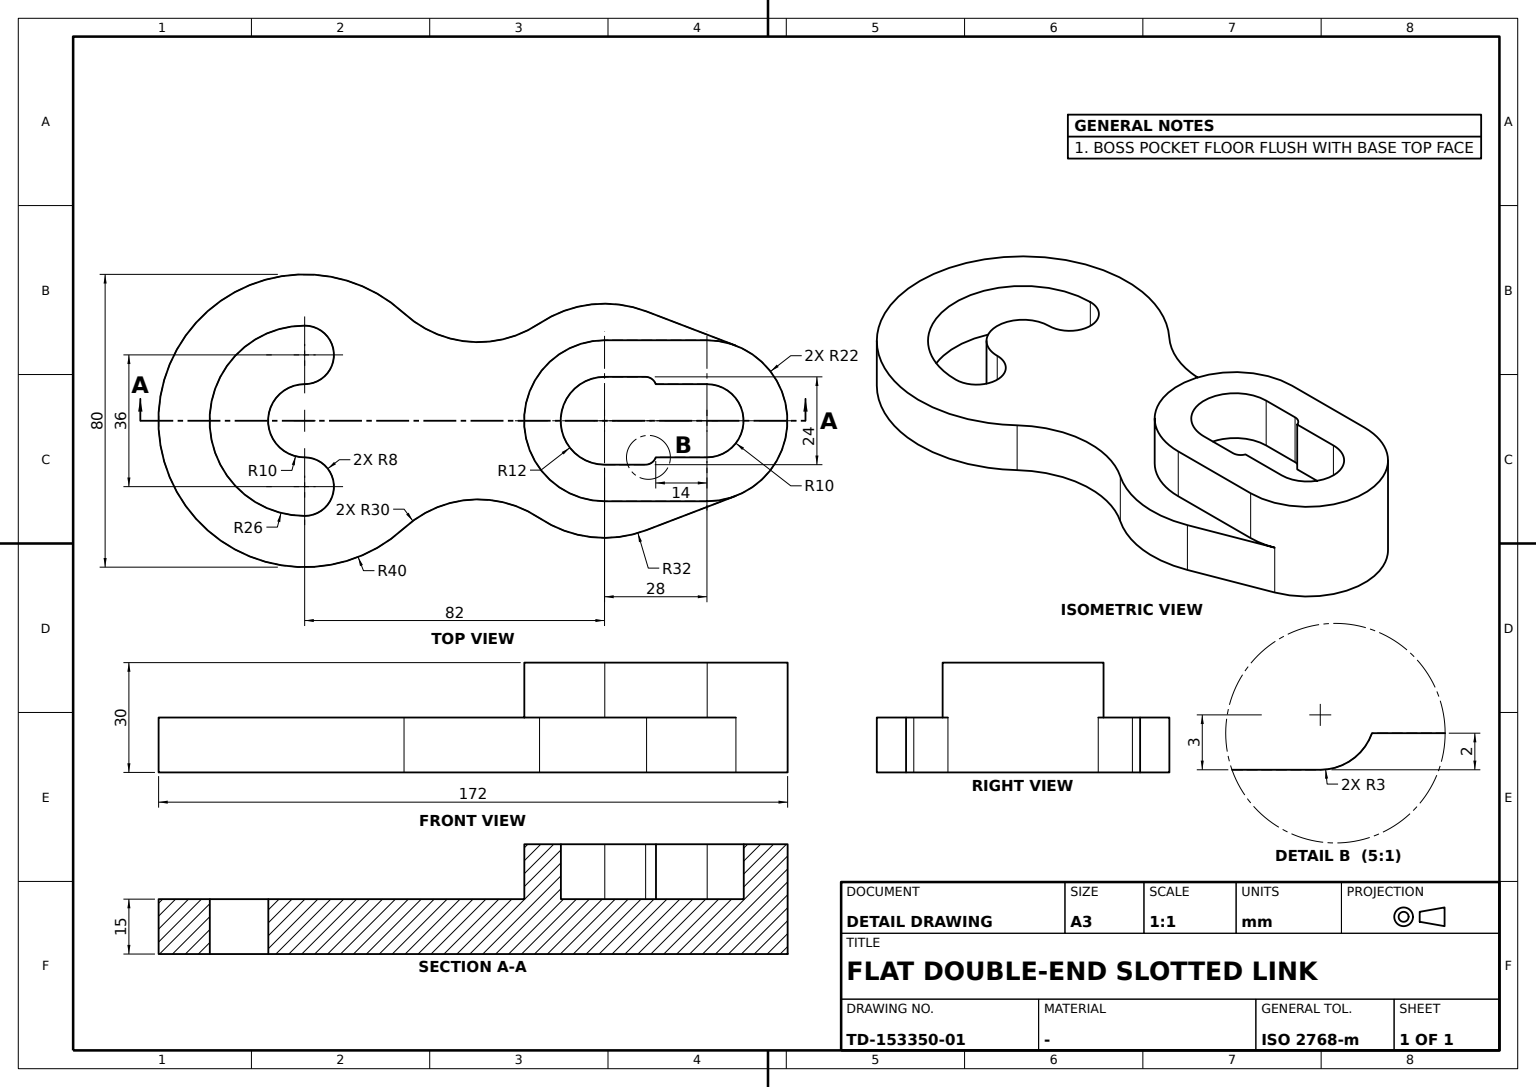
CATIA V5 part; units mm, degrees
sketch "Sketch1" plane through (0, 0, 0) normal (0, 0, 1) x (1, 0, 0)
  arc A0 (-29.4135, 27.108) -> (29.4135, 27.108) centre (0, 0) ccw
  arc A1 (26.5671, 64.1621) -> (29.8896, 93.4286) centre (0, 82) ccw
  point P0 (0, 82)
  arc A2 (26.5671, 64.1621) -> (29.4135, 27.108) centre (51.4737, 47.439) ccw
  arc A3 (-29.4135, 27.108) -> (-26.5671, 64.1621) centre (-51.4737, 47.439) ccw
  arc A4 (20.5491, 117.8571) -> (-20.5491, 117.8571) centre (0, 110) ccw
  point P1 (0, 110)
  line L0 (29.8896, 93.4286) -> (20.5491, 117.8571)
  line L1 (-29.8896, 93.4286) -> (-20.5491, 117.8571)
  point P2 (-29.8896, 93.4286)
  arc A5 (-29.8896, 93.4286) -> (-26.5671, 64.1621) centre (0, 82) ccw
  arc A6 (-18, 0) -> (18, 0) centre (0, 0) ccw construction
  point P3 (0, 0)
  point P4 (-18, 0)
  point P5 (18, 0)
  arc A7 (-26, 0) -> (-10, 0) centre (-18, 0) cw
  arc A8 (10, 0) -> (26, 0) centre (18, 0) cw
  arc A9 (-10, 0) -> (10, 0) centre (0, 0) ccw
  arc A10 (26, 0) -> (-26, 0) centre (0, 0) cw
  dimension "radius A0" = 40
  dimension "radius A1" = 32
  dimension "distance x axis P0" = 82
  dimension "radius A2" = 30
  dimension "radius A3" = 30
  dimension "radius A4" = 22
  dimension "distance P0 P1" = 28
  dimension "radius A8" = 8
  dimension "distance P5 y axis" = 18
  dimension "distance y axis P4" = 18
  constraint coincidence P0 y-axis
  constraint coincidence P1 y-axis
  constraint coincidence P2 A1
  constraint coincidence A1 A5
  constraint coincidence P3 x-axis
  constraint coincidence P4 x-axis
  constraint coincidence P5 x-axis
  constraint tangency A2 A0
  constraint tangency A2 A1
  constraint tangency A3 A0
  constraint tangency A3 A1
  constraint tangency L0 A4
  constraint tangency L0 A1
  constraint tangency L1 A4
  constraint tangency L1 A1
  constraint tangency A9 A8
  constraint tangency A8 A10
  constraint tangency A10 A7
  constraint tangency A7 A9
  constraint concentricity A9 P3
  constraint concentricity A10 P3
extrude "Pad1" add sketch "Sketch1" against normal blind 15
sketch "Sketch2" plane through (0, 0, 0) normal (0, 0, 1) x (1, 0, 0)
  line L0 (0, 110) -> (0, 82) construction
  point P0 (0, 110)
  line L1 (22, 110) -> (22, 82)
  line L2 (-22, 82) -> (-22, 110)
  arc A0 (22, 82) -> (-22, 82) centre (0, 82) cw
  arc A1 (-22, 110) -> (22, 110) centre (0, 110) cw
  arc A2 (20.5491, 117.8571) -> (-20.5491, 117.8571) centre (0, 110) ccw construction
  arc A3 (-12, 82) -> (12, 82) centre (0, 82) ccw
  arc A4 (10, 110) -> (-10, 110) centre (0, 110) ccw
  line L3 (10, 110) -> (10, 96)
  point P1 (10, 110)
  point P2 (10, 96)
  line L4 (12, 82) -> (12, 93.1716)
  point P3 (12, 82)
  point P4 (12, 93.1716)
  arc A5 (12, 93.1716) -> (10, 96) centre (9, 93.1716) ccw
  point P5 (-12, 93.1716)
  point P6 (-12, 82)
  line L5 (-12, 82) -> (-12, 93.1716)
  point P7 (-10, 96)
  arc A6 (-12, 93.1716) -> (-10, 96) centre (-9, 93.1716) cw
  point P8 (-10, 110)
  line L6 (-10, 110) -> (-10, 96)
  point P9 (12, 82)
  dimension "radius A1" = 22
  dimension "length L0" = 28
  dimension "radius A0" = 22
  dimension "radius A3" = 12
  dimension "radius A4" = 10
  dimension "length L3" = 14
  dimension "radius A5" = 3
  constraint coincidence P0 y-axis
  constraint coincidence P3 A3
  constraint coincidence L4 P9
  constraint coincidence P3 P9
  constraint vertical L0 y-axis
  constraint tangency A0 L1
  constraint tangency A1 L1
  constraint tangency A0 L2
  constraint tangency A1 L2
  constraint tangency L3 A4
  constraint tangency L4 A3
  constraint tangency A5 L4
  constraint concentricity A1 A2
  constraint parallelism L3 L0
  constraint parallelism L4 L0
  constraint symmetry P4 P5 L0
  constraint symmetry P3 P6 L0
  constraint symmetry L4 L5 L0
  constraint symmetry P2 P7 L0
  constraint symmetry A5 A6 L0
  constraint symmetry P1 P8 L0
  constraint symmetry L3 L6 L0
extrude "Pad2" add sketch "Sketch2" along normal blind 15
